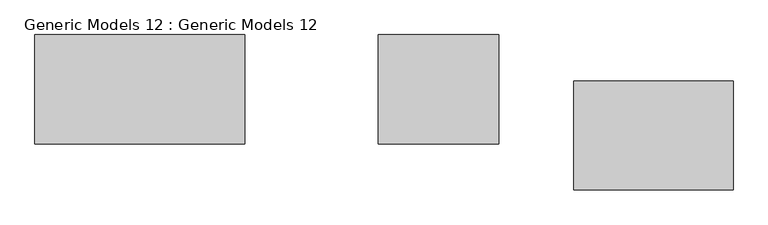
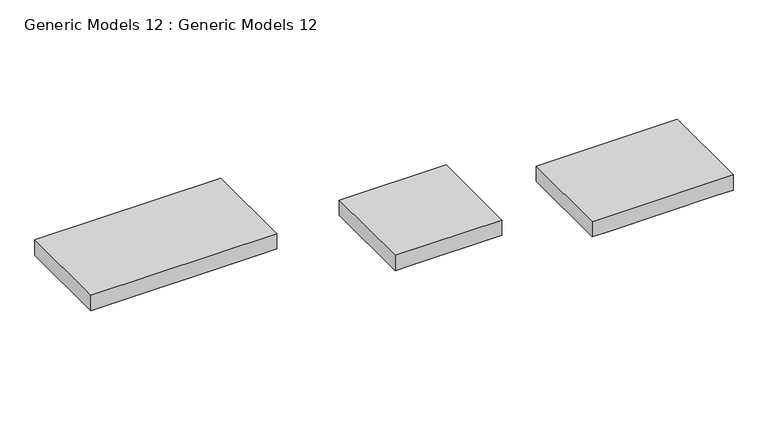
"""IFC4 building model written with IfcOpenShell, lengths in millimetres: proxy geometry, Generic Models 12 : Generic Models 12."""

from ifc_helpers import new_model, si_unit, frame, origin, place, context, project, spatial, polyline, outline, extrude, source, transform, mapped, element, save


def generic_models_12_generic_models_12_6034f315(model_context):
    return source(origin(), model_context, "Body", "SweptSolid", [
        extrude(outline(polyline([(5238.75, -37558.7645004), (5238.75, -37406.3645004), (5238.75, -36377.6645004), (5238.75, -36225.2645004), (5391.15, -36225.2645004), (5391.15, -37558.7645004), (5238.75, -37558.7645004)])), frame((0.0, 4709.3972085, 0.0), z_axis=(0.0, 1.0, 0.0), x_axis=(0.0, 0.0, 1.0)), (0.0, 0.0, 1.0), 914.4),
        extrude(outline(polyline([(5238.75, -39197.0645004), (5238.75, -39044.6645004), (5238.75, -38187.4145004), (5391.15, -38187.4145004), (5391.15, -39197.0645004), (5238.75, -39197.0645004)])), frame((0.0, 5096.8256148, 0.0), z_axis=(0.0, 1.0, 0.0), x_axis=(0.0, 0.0, 1.0)), (0.0, 0.0, 1.0), 914.4),
        extrude(outline(polyline([(5848.35, -40314.6645004), (6000.75, -40314.6645004), (6000.75, -42073.6145004), (5848.35, -42073.6145004), (5848.35, -40467.0645004), (5848.35, -40314.6645004)])), frame((0.0, 5096.8256148, 0.0), z_axis=(0.0, 1.0, 0.0), x_axis=(0.0, 0.0, 1.0)), (0.0, 0.0, 1.0), 914.4),
    ])


if __name__ == "__main__":
    model = new_model("IFC4")
    model_context = context("Model", 3, world=origin())
    ifc_project = project(units=[si_unit("LENGTHUNIT", "METRE", prefix="MILLI")], contexts=[model_context])
    site = spatial("IfcSite", under=ifc_project)
    building = spatial("IfcBuilding", under=site)
    placement = place(None, origin())
    generic_models_12_generic_models_12_shape = generic_models_12_generic_models_12_6034f315(model_context)
    element("IfcBuildingElementProxy", 1, Name="Generic Models 12 : Generic Models 12", ObjectType="Generic Models 12 : Generic Models 12", at=placement, inside=building, context=model_context, shape_type="MappedRepresentation", body=[
        mapped(generic_models_12_generic_models_12_shape, transform((0.0, 0.0, 0.0), x_axis=(1.0, 0.0, 0.0), y_axis=(0.0, 1.0, 0.0), z_axis=(0.0, 0.0, 1.0))),
    ])
    save(model, "model.ifc")
